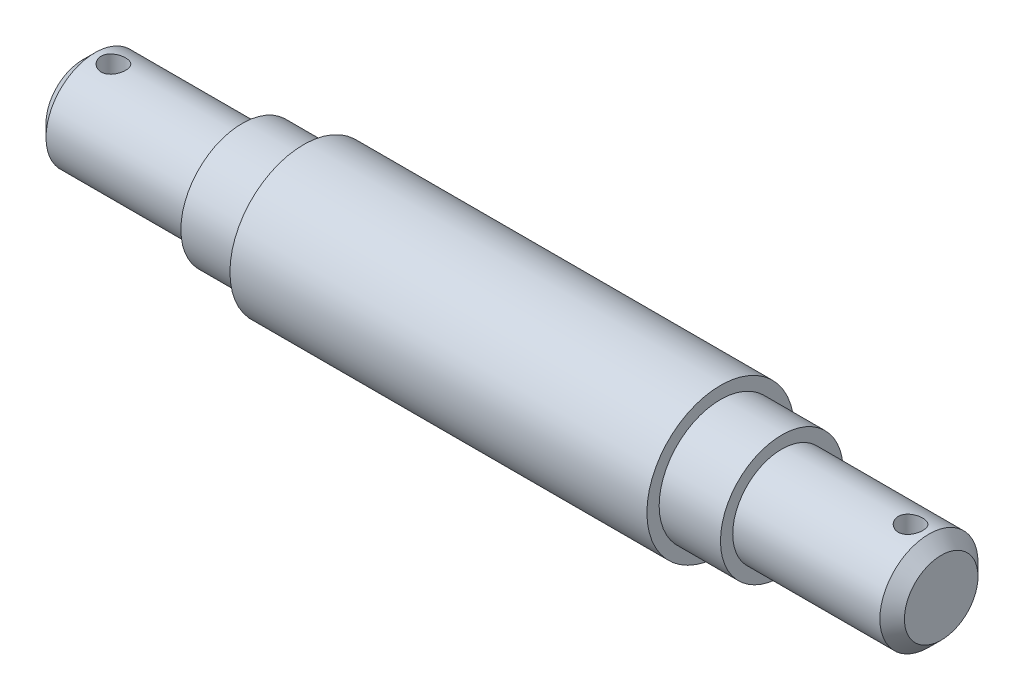
from build123d import *

# Parameters (mm, degrees)
CROSS_HOLE_2_END_1_SKETCH_R = 1
CROSS_HOLE_2_END_1_DEPTH    = 5
CROSS_HOLE_2_END_2_SKETCH_R = 1
CROSS_HOLE_2_END_2_DEPTH    = 11.5
END_CHAMFER_1X45_SIZE       = 1


with BuildPart() as part:
    # Shaft Profile Sketch → Stepped Shaft Body (revolve)
    with BuildSketch(Plane.XY, mode=Mode.PRIVATE) as stepped_shaft_body_sk:
        Polygon((0, 0), (70, 0), (70, -4), (57, -4), (57, -5), (52, -5), (52, -6), (18, -6), (18, -5), (13, -5), (13, -4), (0, -4), align=None)
    revolve(stepped_shaft_body_sk.sketch.rotate(Axis((0, 0, 0), (1, 0, 0)), 270), axis=Axis((0, 0, 0), (1, 0, 0)))

    # Cross Hole Ø2 End 1 Sketch → Cross Hole Ø2 End 1 (cut, symmetric)
    with BuildSketch(Plane(origin=(0, 0, 0), x_dir=(1, 0, 0), z_dir=(0, 1, 0))):
        with Locations(Location((2.5, 0, 0), (0, 0, 270))):
            Circle(CROSS_HOLE_2_END_1_SKETCH_R)
    extrude(amount=CROSS_HOLE_2_END_1_DEPTH, both=True, mode=Mode.SUBTRACT)

    # Cross Hole Ø2 End 2 Sketch → Cross Hole Ø2 End 2 (cut, symmetric)
    with BuildSketch(Plane(origin=(0, 0, 0), x_dir=(1, 0, 0), z_dir=(0, 1, 0))):
        with Locations(Location((67.5, 0, 0), (0, 0, 270))):
            Circle(CROSS_HOLE_2_END_2_SKETCH_R)
    extrude(amount=CROSS_HOLE_2_END_2_DEPTH, both=True, mode=Mode.SUBTRACT)

    # End Chamfer 1x45°
    end_chamfer_1x45_edges = [part.edges().sort_by_distance(p)[0] for p in [
        (70, 0, -4),
        (0, 0, -4),
    ]]
    chamfer(end_chamfer_1x45_edges, length=END_CHAMFER_1X45_SIZE)


solid = part.part
